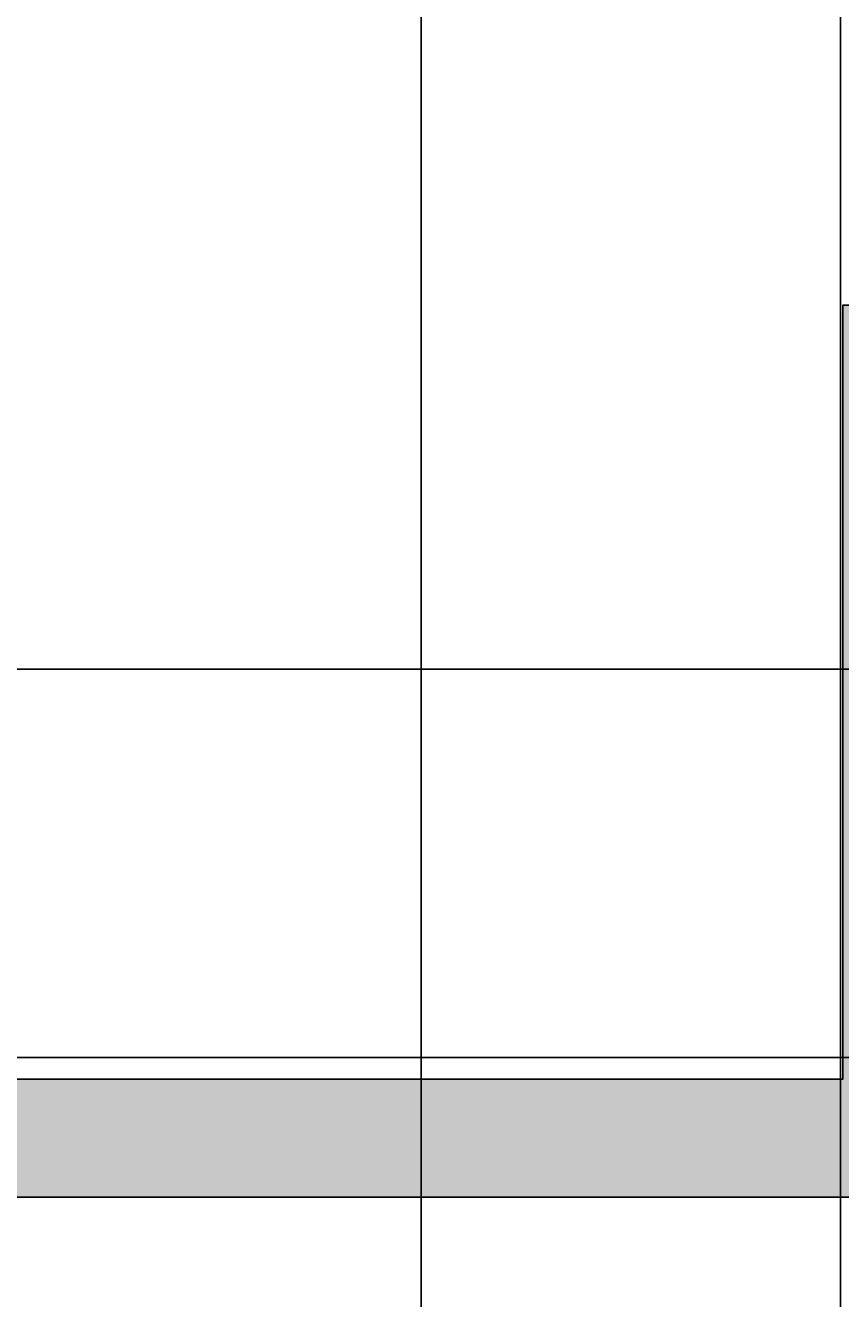
# Model space of a CAD drawing. Units: millimetres. Extents: x -11 to 280, y -4 to 208.
# Tile 13 of 55: x 67 to 91, y 126 to 164. Entities that reach past the tile are written whole.
import ezdxf

# ---------------------------------------------------------------- set-up
doc = ezdxf.new("R2010")
doc.units = ezdxf.units.MM
doc.layers.add('M-DIMS', color=2, linetype='Continuous', lineweight=18)
doc.layers.add('M-HYDR-SUCT', color=7, linetype='Continuous', lineweight=25)
doc.layers.add('M-HYDR-SUCT-PATT', color=221, linetype='Continuous', lineweight=13, true_color=0xff7fdf)
doc.styles.get("Standard").update_dxf_attribs({"font": 'arial.ttf'})
doc.dimstyles.get("Standard").update_dxf_attribs({"dimtxt": 0.18, "dimasz": 0.18, "dimexe": 0.18, "dimexo": 0.0625, "dimgap": 0.09, "dimtad": 0, "dimtih": 1, "dimtoh": 1, "dimdec": 4, "dimzin": 0, "dimdsep": 46, "dimtxsty": 'Standard', "dimcen": 0.09, "dimadec": 0, "dimazin": 0, "dimtfac": 1, "dimtdec": 4, "dimtofl": 0, "dimtmove": 0, "dimatfit": 3, "dimfxl": 1, "dimtolj": 1, "dimtzin": 0, "dimarcsym": 0})

# ---------------------------------------------------------------- blocks, each defined once
blk = doc.blocks.new('*D5')
at = {"layer": 'Defpoints', "color": 0, "transparency": 16777216}
for p in [(24.759, 192.645), (-10.087, 11.435), (261.686, 11.435)]:
    blk.add_point(p, dxfattribs=at)
at = {"layer": 'M-DIMS', "color": 0, "lineweight": -2, "transparency": 16777216}
for p, q in [((24.696, 192.645), (-10.267, 192.645)), ((-10.087, 192.465), (-10.087, 102.222)), ((-10.087, 11.615), (-10.087, 101.858)), ((261.624, 11.435), (-10.267, 11.435))]:
    blk.add_line(p, q, dxfattribs=at)
at = {"layer": 'M-DIMS', "color": 0, "transparency": 16777216}
for points in [[(-10.117, 192.465), (-10.057, 192.465), (-10.087, 192.645)], [(-10.117, 11.615), (-10.057, 11.615), (-10.087, 11.435)]]:
    blk.add_solid(points, dxfattribs=at)
at = {"layer": 'M-DIMS', "color": 0, "transparency": 16777216, "insert": (-10.087, 102.04), "char_height": 0.18, "attachment_point": 5}
blk.add_mtext('\\A1;181.2', dxfattribs=at)
blk = doc.blocks.new('*D9')
at = {"layer": 'Defpoints', "color": 0, "transparency": 16777216}
for p in [(78.827, 207.495), (31.006, 98.021), (78.827, 98.149)]:
    blk.add_point(p, dxfattribs=at)
at = {"layer": 'M-DIMS', "color": 0, "lineweight": -2, "transparency": 16777216}
for p, q in [((31.006, 98.084), (31.006, 207.675)), ((31.186, 207.495), (54.52, 207.495)), ((78.647, 207.495), (55.313, 207.495)), ((78.827, 98.212), (78.827, 207.675))]:
    blk.add_line(p, q, dxfattribs=at)
at = {"layer": 'M-DIMS', "color": 0, "transparency": 16777216}
for points in [[(31.186, 207.525), (31.186, 207.465), (31.006, 207.495)], [(78.647, 207.525), (78.647, 207.465), (78.827, 207.495)]]:
    blk.add_solid(points, dxfattribs=at)
at = {"layer": 'M-DIMS', "color": 0, "transparency": 16777216, "insert": (54.917, 207.495), "char_height": 0.18, "attachment_point": 5}
blk.add_mtext('\\A1;47.82', dxfattribs=at)
blk = doc.blocks.new('*D11')
at = {"layer": 'Defpoints', "color": 0, "transparency": 16777216}
for p in [(118.514, 207.495), (91.3, 98.149), (118.514, 96.485)]:
    blk.add_point(p, dxfattribs=at)
at = {"layer": 'M-DIMS', "color": 0, "lineweight": -2, "transparency": 16777216}
for p, q in [((91.3, 98.212), (91.3, 207.675)), ((91.48, 207.495), (104.442, 207.495)), ((118.334, 207.495), (105.372, 207.495)), ((118.514, 96.547), (118.514, 207.675))]:
    blk.add_line(p, q, dxfattribs=at)
at = {"layer": 'M-DIMS', "color": 0, "transparency": 16777216}
for points in [[(91.48, 207.525), (91.48, 207.465), (91.3, 207.495)], [(118.334, 207.525), (118.334, 207.465), (118.514, 207.495)]]:
    blk.add_solid(points, dxfattribs=at)
at = {"layer": 'M-DIMS', "color": 0, "transparency": 16777216, "insert": (104.907, 207.495), "char_height": 0.18, "attachment_point": 5}
blk.add_mtext('\\A1;27.214', dxfattribs=at)
blk = doc.blocks.new('*D14')
at = {"layer": 'Defpoints', "color": 0, "transparency": 16777216}
for p in [(-10.087, 144.661), (205.531, 144.661), (226.511, 133.123)]:
    blk.add_point(p, dxfattribs=at)
at = {"layer": 'M-DIMS', "color": 0, "lineweight": -2, "transparency": 16777216}
for p, q in [((205.469, 144.661), (-10.267, 144.661)), ((-10.087, 144.481), (-10.087, 139.074)), ((-10.087, 133.303), (-10.087, 138.71)), ((226.448, 133.123), (-10.267, 133.123))]:
    blk.add_line(p, q, dxfattribs=at)
at = {"layer": 'M-DIMS', "color": 0, "transparency": 16777216}
for points in [[(-10.117, 144.481), (-10.057, 144.481), (-10.087, 144.661)], [(-10.117, 133.303), (-10.057, 133.303), (-10.087, 133.123)]]:
    blk.add_solid(points, dxfattribs=at)
at = {"layer": 'M-DIMS', "color": 0, "transparency": 16777216, "insert": (-10.087, 138.892), "char_height": 0.18, "attachment_point": 5}
blk.add_mtext('\\A1;11.538', dxfattribs=at)

msp = doc.modelspace()

# ---------------------------------------------------------------- hatches: boundary and pattern name
at = {"layer": 'M-HYDR-SUCT-PATT'}
h = msp.add_hatch(color=256, dxfattribs=at)
h.set_gradient(color1=(255, 127, 223), color2=(255, 127, 223), tint=1, name='INVCYLINDER')
h.paths.add_polyline_path([(91.3629, 155.4768), (91.3629, 132.4768), (58.3629, 132.4768), (58.3629, 153.9768), (54.8629, 153.9768), (54.8629, 128.9768), (94.8629, 128.9768), (94.8629, 151.9768), (205.5315, 151.9768), (205.5315, 155.4768)])
h.paths.add_polyline_path([(91.3, 114.9452, 1), (78.8273, 114.9452), (78.8273, 108.8141), (42.6453, 108.8141), (42.6453, 153.9768), (39.1453, 153.9768), (39.1453, 105.3141), (78.8273, 105.3141), (78.8273, 98.1491, 1), (91.3, 98.1491), (91.3, 105.3141), (95.5776, 105.3141), (95.5776, 108.8141), (91.3, 108.8141)])
h.paths.add_polyline_path([(228.7, 138.4081), (232.2, 138.4081), (232.2, 144.6609), (228.7, 144.6609)])
h.paths.add_polyline_path([(253.1005, 151.9768, 1), (253.1005, 155.4768), (252.6001, 155.4768), (253.5249, 153.991, -0.1401047), (253.6005, 153.7268, -0.7542249), (252.676, 153.4626), (251.4221, 155.4768), (236.9353, 155.4768), (236.9353, 151.9768)])
h.paths.add_polyline_path([(30.8182, 40.7626), (30.8182, 36.7626), (60.8182, 36.7626), (60.8182, 40.7626)])

# ---------------------------------------------------------------- linework, layer by layer
at = {"layer": 'M-HYDR-SUCT'}
for points in [[(58.3629, 153.9768), (58.3629, 132.4768), (91.3629, 132.4768), (91.3629, 155.4768), (205.5315, 155.4768)], [(54.8629, 153.9768), (54.8629, 128.9768), (94.8629, 128.9768), (94.8629, 151.9768), (205.5315, 151.9768)]]:
    msp.add_lwpolyline(points, dxfattribs=at)

# ---------------------------------------------------------------- dimensions: what is measured, and where the dimension line sits
at = {"layer": 'M-DIMS'}
for base, p1, p2, override, picture, middle in [((78.8273, 207.495), (31.0059, 98.0213), (78.8273, 98.1491), {"dimdec": 2, "dimlfac": 1, "dimrnd": 0, "dimzin": 0, "dimdsep": 46, "dimlunit": 2}, '*D9', (54.9166, 207.495)), ((118.5137, 207.495), (91.3, 98.1491), (118.5137, 96.4849), {"dimdec": 3, "dimlfac": 1, "dimrnd": 0, "dimzin": 0, "dimdsep": 46, "dimlunit": 2}, '*D11', (104.9068, 207.495))]:
    dim = msp.add_linear_dim(base=base, p1=p1, p2=p2, dimstyle='Standard', override=override, dxfattribs=at)
    dim.commit()
    dim.dimension.update_dxf_attribs({"geometry": picture, "text_midpoint": middle})
for base, p1, p2, override, picture, middle in [((-10.0865, 11.4346), (24.7588, 192.645), (261.6863, 11.4346), {"dimdec": 1, "dimlfac": 1, "dimrnd": 0, "dimzin": 0, "dimdsep": 46, "dimlunit": 2}, '*D5', (-10.0865, 102.0398)), ((-10.0865, 144.6609), (226.5106, 133.1228), (205.5315, 144.6609), {"dimdec": 3, "dimlfac": 1, "dimrnd": 0, "dimzin": 0, "dimdsep": 46, "dimlunit": 2}, '*D14', (-10.0865, 138.8918))]:
    dim = msp.add_linear_dim(base=base, p1=p1, p2=p2, angle=90, dimstyle='Standard', override=override, dxfattribs=at)
    dim.commit()
    dim.dimension.update_dxf_attribs({"geometry": picture, "text_midpoint": middle})

doc.saveas('drawing.dxf')
